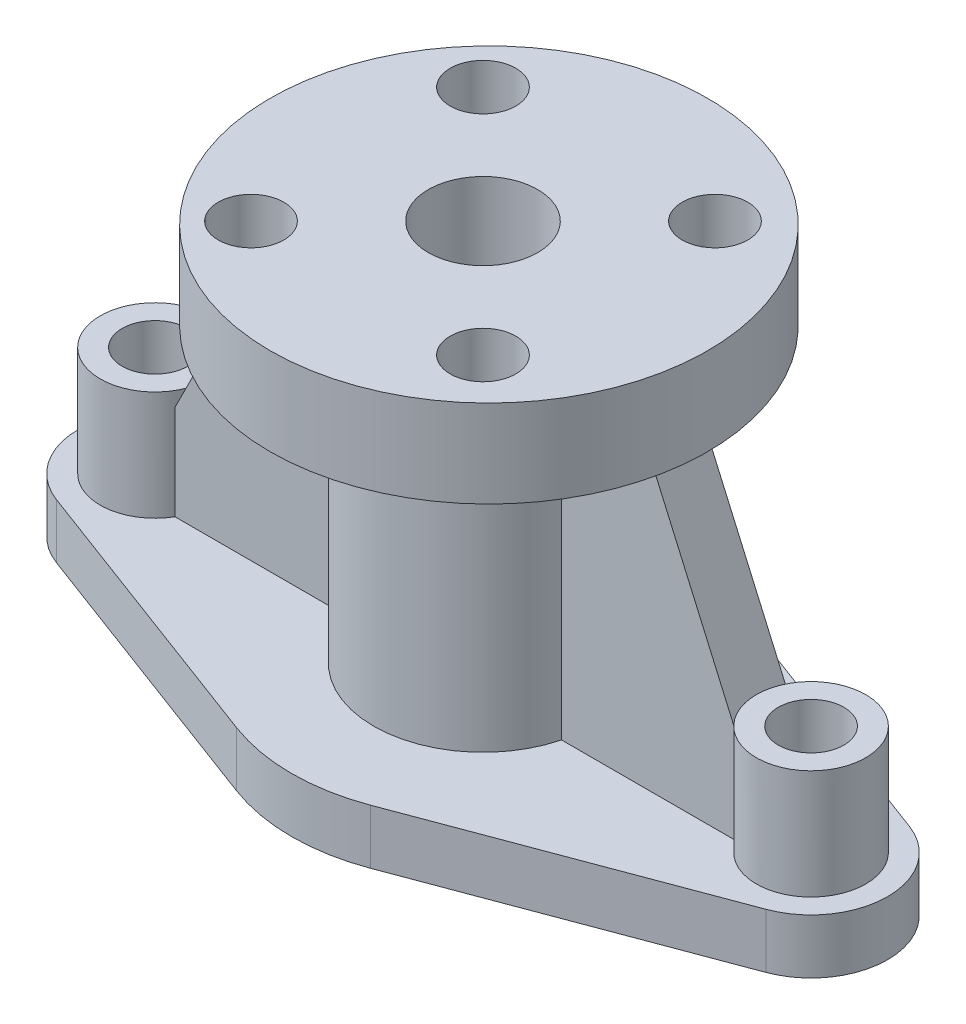
ISO-10303-21;
HEADER;
FILE_DESCRIPTION(('STEP AP214'),'2;1');
FILE_NAME('part.step','',(''),(''),'','','');
FILE_SCHEMA(('AUTOMOTIVE_DESIGN { 1 0 10303 214 1 1 1 1 }'));
ENDSEC;
DATA;
#1=APPLICATION_CONTEXT('core data for automotive mechanical design processes');
#2=APPLICATION_PROTOCOL_DEFINITION('international standard','automotive_design',2000,#1);
#3=PRODUCT_CONTEXT('',#1,'mechanical');
#4=PRODUCT('Part','Part','',(#3));
#5=PRODUCT_RELATED_PRODUCT_CATEGORY('part','',(#4));
#6=PRODUCT_DEFINITION_FORMATION('','',#4);
#7=PRODUCT_DEFINITION_CONTEXT('part definition',#1,'design');
#8=PRODUCT_DEFINITION('design','',#6,#7);
#9=PRODUCT_DEFINITION_SHAPE('','',#8);
#10=(LENGTH_UNIT() NAMED_UNIT(*) SI_UNIT(.MILLI.,.METRE.));
#11=(NAMED_UNIT(*) PLANE_ANGLE_UNIT() SI_UNIT($,.RADIAN.));
#12=(NAMED_UNIT(*) SI_UNIT($,.STERADIAN.) SOLID_ANGLE_UNIT());
#13=UNCERTAINTY_MEASURE_WITH_UNIT(LENGTH_MEASURE(1.E-05),#10,'distance_accuracy_value','');
#14=(GEOMETRIC_REPRESENTATION_CONTEXT(3) GLOBAL_UNCERTAINTY_ASSIGNED_CONTEXT((#13)) GLOBAL_UNIT_ASSIGNED_CONTEXT((#10,
#11,#12)) REPRESENTATION_CONTEXT('',''));
#15=CARTESIAN_POINT('',(0.,0.,0.));
#16=DIRECTION('',(0.,0.,1.));
#17=DIRECTION('',(1.,0.,0.));
#18=AXIS2_PLACEMENT_3D('',#15,#16,#17);
#19=CARTESIAN_POINT('',(0.,-0.002000000000002,0.));
#20=DIRECTION('',(0.,1.,0.));
#21=DIRECTION('',(0.,0.,1.));
#22=AXIS2_PLACEMENT_3D('',#19,#20,#21);
#23=CYLINDRICAL_SURFACE('',#22,20.);
#24=DIRECTION('',(0.,1.,0.));
#25=VECTOR('',#24,1.);
#26=CARTESIAN_POINT('',(19.3649167310371,-0.002000000000002,-5.));
#27=LINE('',#26,#25);
#28=CARTESIAN_POINT('',(19.3649167310371,10.,-5.));
#29=VERTEX_POINT('',#28);
#30=CARTESIAN_POINT('',(19.3649167310371,64.,-5.));
#31=VERTEX_POINT('',#30);
#32=EDGE_CURVE('E191',#29,#31,#27,.T.);
#33=ORIENTED_EDGE('',*,*,#32,.F.);
#34=CARTESIAN_POINT('',(0.,10.,0.));
#35=DIRECTION('',(0.,1.,0.));
#36=DIRECTION('',(0.,0.,1.));
#37=AXIS2_PLACEMENT_3D('',#34,#35,#36);
#38=CIRCLE('',#37,20.);
#39=CARTESIAN_POINT('',(-19.3649167310371,10.,-5.));
#40=VERTEX_POINT('',#39);
#41=EDGE_CURVE('E265',#29,#40,#38,.T.);
#42=ORIENTED_EDGE('',*,*,#41,.T.);
#43=DIRECTION('',(0.,1.,0.));
#44=VECTOR('',#43,1.);
#45=CARTESIAN_POINT('',(-19.3649167310371,-0.002000000000002,-5.));
#46=LINE('',#45,#44);
#47=CARTESIAN_POINT('',(-19.3649167310371,64.,-5.));
#48=VERTEX_POINT('',#47);
#49=EDGE_CURVE('E228',#48,#40,#46,.F.);
#50=ORIENTED_EDGE('',*,*,#49,.F.);
#51=CARTESIAN_POINT('',(0.,64.,0.));
#52=DIRECTION('',(0.,-1.,0.));
#53=DIRECTION('',(0.,0.,-1.));
#54=AXIS2_PLACEMENT_3D('',#51,#52,#53);
#55=CIRCLE('',#54,20.);
#56=EDGE_CURVE('E261',#48,#31,#55,.T.);
#57=ORIENTED_EDGE('',*,*,#56,.T.);
#58=EDGE_LOOP('',(#33,#42,#50,#57));
#59=FACE_BOUND('',#58,.T.);
#60=ADVANCED_FACE('F39',(#59),#23,.T.);
#61=CARTESIAN_POINT('',(-60.,10.,0.));
#62=DIRECTION('',(0.,-1.,0.));
#63=DIRECTION('',(0.,0.,-1.));
#64=AXIS2_PLACEMENT_3D('',#61,#62,#63);
#65=CYLINDRICAL_SURFACE('',#64,14.);
#66=DIRECTION('',(0.,-1.,0.));
#67=VECTOR('',#66,1.);
#68=CARTESIAN_POINT('',(-64.9,10.,13.1144957966366));
#69=LINE('',#68,#67);
#70=CARTESIAN_POINT('',(-64.9,10.,13.1144957966366));
#71=VERTEX_POINT('',#70);
#72=CARTESIAN_POINT('',(-64.9,0.,13.1144957966366));
#73=VERTEX_POINT('',#72);
#74=EDGE_CURVE('E11',#71,#73,#69,.T.);
#75=ORIENTED_EDGE('',*,*,#74,.F.);
#76=CARTESIAN_POINT('',(-60.,10.,0.));
#77=DIRECTION('',(0.,1.,0.));
#78=DIRECTION('',(0.,0.,1.));
#79=AXIS2_PLACEMENT_3D('',#76,#77,#78);
#80=CIRCLE('',#79,14.);
#81=CARTESIAN_POINT('',(-64.9,10.,-13.1144957966366));
#82=VERTEX_POINT('',#81);
#83=EDGE_CURVE('E288',#82,#71,#80,.T.);
#84=ORIENTED_EDGE('',*,*,#83,.F.);
#85=DIRECTION('',(0.,-1.,0.));
#86=VECTOR('',#85,1.);
#87=CARTESIAN_POINT('',(-64.9,10.,-13.1144957966366));
#88=LINE('',#87,#86);
#89=CARTESIAN_POINT('',(-64.9,0.,-13.1144957966366));
#90=VERTEX_POINT('',#89);
#91=EDGE_CURVE('E303',#82,#90,#88,.T.);
#92=ORIENTED_EDGE('',*,*,#91,.T.);
#93=CARTESIAN_POINT('',(-60.,0.,0.));
#94=DIRECTION('',(0.,1.,0.));
#95=DIRECTION('',(0.,0.,1.));
#96=AXIS2_PLACEMENT_3D('',#93,#94,#95);
#97=CIRCLE('',#96,14.);
#98=EDGE_CURVE('E280',#90,#73,#97,.T.);
#99=ORIENTED_EDGE('',*,*,#98,.T.);
#100=EDGE_LOOP('',(#75,#84,#92,#99));
#101=FACE_BOUND('',#100,.T.);
#102=ADVANCED_FACE('F41',(#101),#65,.T.);
#103=CARTESIAN_POINT('',(-64.9,10.,13.1144957966366));
#104=DIRECTION('',(0.35,0.,-0.93674969975976));
#105=DIRECTION('',(-0.93674969975976,0.,-0.35));
#106=AXIS2_PLACEMENT_3D('',#103,#104,#105);
#107=PLANE('',#106);
#108=DIRECTION('',(0.93674969975976,0.,0.35));
#109=VECTOR('',#108,1.);
#110=CARTESIAN_POINT('',(-64.9,0.,13.1144957966366));
#111=LINE('',#110,#109);
#112=CARTESIAN_POINT('',(-12.25,0.,32.7862394915916));
#113=VERTEX_POINT('',#112);
#114=EDGE_CURVE('E304',#73,#113,#111,.T.);
#115=ORIENTED_EDGE('',*,*,#114,.T.);
#116=DIRECTION('',(0.,-1.,0.));
#117=VECTOR('',#116,1.);
#118=CARTESIAN_POINT('',(-12.25,10.,32.7862394915916));
#119=LINE('',#118,#117);
#120=CARTESIAN_POINT('',(-12.25,10.,32.7862394915916));
#121=VERTEX_POINT('',#120);
#122=EDGE_CURVE('E48',#121,#113,#119,.T.);
#123=ORIENTED_EDGE('',*,*,#122,.F.);
#124=DIRECTION('',(0.93674969975976,0.,0.35));
#125=VECTOR('',#124,1.);
#126=CARTESIAN_POINT('',(-64.9,10.,13.1144957966366));
#127=LINE('',#126,#125);
#128=EDGE_CURVE('E286',#71,#121,#127,.T.);
#129=ORIENTED_EDGE('',*,*,#128,.F.);
#130=ORIENTED_EDGE('',*,*,#74,.T.);
#131=EDGE_LOOP('',(#115,#123,#129,#130));
#132=FACE_BOUND('',#131,.T.);
#133=ADVANCED_FACE('F362',(#132),#107,.F.);
#134=CARTESIAN_POINT('',(0.,10.,0.));
#135=DIRECTION('',(0.,-1.,0.));
#136=DIRECTION('',(0.,0.,-1.));
#137=AXIS2_PLACEMENT_3D('',#134,#135,#136);
#138=CYLINDRICAL_SURFACE('',#137,35.);
#139=CARTESIAN_POINT('',(0.,0.,0.));
#140=DIRECTION('',(0.,1.,0.));
#141=DIRECTION('',(0.,0.,1.));
#142=AXIS2_PLACEMENT_3D('',#139,#140,#141);
#143=CIRCLE('',#142,35.);
#144=CARTESIAN_POINT('',(12.25,0.,32.7862394915916));
#145=VERTEX_POINT('',#144);
#146=EDGE_CURVE('E310',#113,#145,#143,.T.);
#147=ORIENTED_EDGE('',*,*,#146,.T.);
#148=DIRECTION('',(0.,-1.,0.));
#149=VECTOR('',#148,1.);
#150=CARTESIAN_POINT('',(12.25,10.,32.7862394915916));
#151=LINE('',#150,#149);
#152=CARTESIAN_POINT('',(12.25,10.,32.7862394915916));
#153=VERTEX_POINT('',#152);
#154=EDGE_CURVE('E335',#153,#145,#151,.T.);
#155=ORIENTED_EDGE('',*,*,#154,.F.);
#156=CARTESIAN_POINT('',(0.,10.,0.));
#157=DIRECTION('',(0.,1.,0.));
#158=DIRECTION('',(0.,0.,1.));
#159=AXIS2_PLACEMENT_3D('',#156,#157,#158);
#160=CIRCLE('',#159,35.);
#161=EDGE_CURVE('E293',#121,#153,#160,.T.);
#162=ORIENTED_EDGE('',*,*,#161,.F.);
#163=ORIENTED_EDGE('',*,*,#122,.T.);
#164=EDGE_LOOP('',(#147,#155,#162,#163));
#165=FACE_BOUND('',#164,.T.);
#166=ADVANCED_FACE('F338',(#165),#138,.T.);
#167=CARTESIAN_POINT('',(64.9,10.,13.1144957966366));
#168=DIRECTION('',(-0.35,0.,-0.93674969975976));
#169=DIRECTION('',(-0.93674969975976,0.,0.35));
#170=AXIS2_PLACEMENT_3D('',#167,#168,#169);
#171=PLANE('',#170);
#172=DIRECTION('',(0.93674969975976,0.,-0.35));
#173=VECTOR('',#172,1.);
#174=CARTESIAN_POINT('',(64.9,0.,13.1144957966366));
#175=LINE('',#174,#173);
#176=CARTESIAN_POINT('',(64.9,0.,13.1144957966366));
#177=VERTEX_POINT('',#176);
#178=EDGE_CURVE('E307',#145,#177,#175,.T.);
#179=ORIENTED_EDGE('',*,*,#178,.T.);
#180=DIRECTION('',(0.,-1.,0.));
#181=VECTOR('',#180,1.);
#182=CARTESIAN_POINT('',(64.9,10.,13.1144957966366));
#183=LINE('',#182,#181);
#184=CARTESIAN_POINT('',(64.9,10.,13.1144957966366));
#185=VERTEX_POINT('',#184);
#186=EDGE_CURVE('E327',#185,#177,#183,.T.);
#187=ORIENTED_EDGE('',*,*,#186,.F.);
#188=DIRECTION('',(0.93674969975976,0.,-0.35));
#189=VECTOR('',#188,1.);
#190=CARTESIAN_POINT('',(64.9,10.,13.1144957966366));
#191=LINE('',#190,#189);
#192=EDGE_CURVE('E291',#153,#185,#191,.T.);
#193=ORIENTED_EDGE('',*,*,#192,.F.);
#194=ORIENTED_EDGE('',*,*,#154,.T.);
#195=EDGE_LOOP('',(#179,#187,#193,#194));
#196=FACE_BOUND('',#195,.T.);
#197=ADVANCED_FACE('F351',(#196),#171,.F.);
#198=CARTESIAN_POINT('',(60.,10.,0.));
#199=DIRECTION('',(0.,-1.,0.));
#200=DIRECTION('',(0.,0.,-1.));
#201=AXIS2_PLACEMENT_3D('',#198,#199,#200);
#202=CYLINDRICAL_SURFACE('',#201,14.);
#203=CARTESIAN_POINT('',(60.,0.,0.));
#204=DIRECTION('',(0.,1.,0.));
#205=DIRECTION('',(0.,0.,1.));
#206=AXIS2_PLACEMENT_3D('',#203,#204,#205);
#207=CIRCLE('',#206,14.);
#208=CARTESIAN_POINT('',(64.9,0.,-13.1144957966367));
#209=VERTEX_POINT('',#208);
#210=EDGE_CURVE('E311',#177,#209,#207,.T.);
#211=ORIENTED_EDGE('',*,*,#210,.T.);
#212=DIRECTION('',(0.,-1.,0.));
#213=VECTOR('',#212,1.);
#214=CARTESIAN_POINT('',(64.9,10.,-13.1144957966367));
#215=LINE('',#214,#213);
#216=CARTESIAN_POINT('',(64.9,10.,-13.1144957966367));
#217=VERTEX_POINT('',#216);
#218=EDGE_CURVE('E328',#217,#209,#215,.T.);
#219=ORIENTED_EDGE('',*,*,#218,.F.);
#220=CARTESIAN_POINT('',(60.,10.,0.));
#221=DIRECTION('',(0.,1.,0.));
#222=DIRECTION('',(0.,0.,1.));
#223=AXIS2_PLACEMENT_3D('',#220,#221,#222);
#224=CIRCLE('',#223,14.);
#225=EDGE_CURVE('E294',#185,#217,#224,.T.);
#226=ORIENTED_EDGE('',*,*,#225,.F.);
#227=ORIENTED_EDGE('',*,*,#186,.T.);
#228=EDGE_LOOP('',(#211,#219,#226,#227));
#229=FACE_BOUND('',#228,.T.);
#230=ADVANCED_FACE('F357',(#229),#202,.T.);
#231=CARTESIAN_POINT('',(64.9,10.,-13.1144957966367));
#232=DIRECTION('',(-0.35,0.,0.93674969975976));
#233=DIRECTION('',(0.93674969975976,0.,0.35));
#234=AXIS2_PLACEMENT_3D('',#231,#232,#233);
#235=PLANE('',#234);
#236=DIRECTION('',(-0.93674969975976,0.,-0.35));
#237=VECTOR('',#236,1.);
#238=CARTESIAN_POINT('',(64.9,0.,-13.1144957966367));
#239=LINE('',#238,#237);
#240=CARTESIAN_POINT('',(12.25,0.,-32.7862394915916));
#241=VERTEX_POINT('',#240);
#242=EDGE_CURVE('E312',#209,#241,#239,.T.);
#243=ORIENTED_EDGE('',*,*,#242,.T.);
#244=DIRECTION('',(0.,-1.,0.));
#245=VECTOR('',#244,1.);
#246=CARTESIAN_POINT('',(12.25,10.,-32.7862394915916));
#247=LINE('',#246,#245);
#248=CARTESIAN_POINT('',(12.25,10.,-32.7862394915916));
#249=VERTEX_POINT('',#248);
#250=EDGE_CURVE('E325',#249,#241,#247,.T.);
#251=ORIENTED_EDGE('',*,*,#250,.F.);
#252=DIRECTION('',(-0.93674969975976,0.,-0.35));
#253=VECTOR('',#252,1.);
#254=CARTESIAN_POINT('',(64.9,10.,-13.1144957966367));
#255=LINE('',#254,#253);
#256=EDGE_CURVE('E300',#217,#249,#255,.T.);
#257=ORIENTED_EDGE('',*,*,#256,.F.);
#258=ORIENTED_EDGE('',*,*,#218,.T.);
#259=EDGE_LOOP('',(#243,#251,#257,#258));
#260=FACE_BOUND('',#259,.T.);
#261=ADVANCED_FACE('F377',(#260),#235,.F.);
#262=CARTESIAN_POINT('',(0.,10.,0.));
#263=DIRECTION('',(0.,-1.,0.));
#264=DIRECTION('',(0.,0.,-1.));
#265=AXIS2_PLACEMENT_3D('',#262,#263,#264);
#266=CYLINDRICAL_SURFACE('',#265,35.);
#267=CARTESIAN_POINT('',(0.,0.,0.));
#268=DIRECTION('',(0.,1.,0.));
#269=DIRECTION('',(0.,0.,1.));
#270=AXIS2_PLACEMENT_3D('',#267,#268,#269);
#271=CIRCLE('',#270,35.);
#272=CARTESIAN_POINT('',(-12.25,0.,-32.7862394915916));
#273=VERTEX_POINT('',#272);
#274=EDGE_CURVE('E314',#241,#273,#271,.T.);
#275=ORIENTED_EDGE('',*,*,#274,.T.);
#276=DIRECTION('',(0.,-1.,0.));
#277=VECTOR('',#276,1.);
#278=CARTESIAN_POINT('',(-12.25,10.,-32.7862394915916));
#279=LINE('',#278,#277);
#280=CARTESIAN_POINT('',(-12.25,10.,-32.7862394915916));
#281=VERTEX_POINT('',#280);
#282=EDGE_CURVE('E318',#281,#273,#279,.T.);
#283=ORIENTED_EDGE('',*,*,#282,.F.);
#284=CARTESIAN_POINT('',(0.,10.,0.));
#285=DIRECTION('',(0.,1.,0.));
#286=DIRECTION('',(0.,0.,1.));
#287=AXIS2_PLACEMENT_3D('',#284,#285,#286);
#288=CIRCLE('',#287,35.);
#289=EDGE_CURVE('E299',#249,#281,#288,.T.);
#290=ORIENTED_EDGE('',*,*,#289,.F.);
#291=ORIENTED_EDGE('',*,*,#250,.T.);
#292=EDGE_LOOP('',(#275,#283,#290,#291));
#293=FACE_BOUND('',#292,.T.);
#294=ADVANCED_FACE('F376',(#293),#266,.T.);
#295=CARTESIAN_POINT('',(-64.9,10.,-13.1144957966366));
#296=DIRECTION('',(0.35,0.,0.93674969975976));
#297=DIRECTION('',(0.93674969975976,0.,-0.35));
#298=AXIS2_PLACEMENT_3D('',#295,#296,#297);
#299=PLANE('',#298);
#300=DIRECTION('',(-0.93674969975976,0.,0.35));
#301=VECTOR('',#300,1.);
#302=CARTESIAN_POINT('',(-64.9,0.,-13.1144957966366));
#303=LINE('',#302,#301);
#304=EDGE_CURVE('E289',#273,#90,#303,.T.);
#305=ORIENTED_EDGE('',*,*,#304,.T.);
#306=ORIENTED_EDGE('',*,*,#91,.F.);
#307=DIRECTION('',(-0.93674969975976,0.,0.35));
#308=VECTOR('',#307,1.);
#309=CARTESIAN_POINT('',(-64.9,10.,-13.1144957966366));
#310=LINE('',#309,#308);
#311=EDGE_CURVE('E301',#281,#82,#310,.T.);
#312=ORIENTED_EDGE('',*,*,#311,.F.);
#313=ORIENTED_EDGE('',*,*,#282,.T.);
#314=EDGE_LOOP('',(#305,#306,#312,#313));
#315=FACE_BOUND('',#314,.T.);
#316=ADVANCED_FACE('F371',(#315),#299,.F.);
#317=CARTESIAN_POINT('',(-60.,10.,0.));
#318=DIRECTION('',(0.,1.,0.));
#319=DIRECTION('',(0.,0.,1.));
#320=AXIS2_PLACEMENT_3D('',#317,#318,#319);
#321=PLANE('',#320);
#322=DIRECTION('',(1.,0.,0.));
#323=VECTOR('',#322,1.);
#324=CARTESIAN_POINT('',(-60.,10.,5.));
#325=LINE('',#324,#323);
#326=CARTESIAN_POINT('',(-51.3397459621556,10.,5.));
#327=VERTEX_POINT('',#326);
#328=CARTESIAN_POINT('',(-19.3649167310371,10.,5.));
#329=VERTEX_POINT('',#328);
#330=EDGE_CURVE('E237',#327,#329,#325,.T.);
#331=ORIENTED_EDGE('',*,*,#330,.F.);
#332=CARTESIAN_POINT('',(-60.,10.,0.));
#333=DIRECTION('',(0.,1.,0.));
#334=DIRECTION('',(0.,0.,1.));
#335=AXIS2_PLACEMENT_3D('',#332,#333,#334);
#336=CIRCLE('',#335,10.);
#337=CARTESIAN_POINT('',(-51.3397459621556,10.,-5.));
#338=VERTEX_POINT('',#337);
#339=EDGE_CURVE('E274',#338,#327,#336,.T.);
#340=ORIENTED_EDGE('',*,*,#339,.F.);
#341=DIRECTION('',(1.,0.,0.));
#342=VECTOR('',#341,1.);
#343=CARTESIAN_POINT('',(-60.,10.,-5.));
#344=LINE('',#343,#342);
#345=EDGE_CURVE('E227',#338,#40,#344,.T.);
#346=ORIENTED_EDGE('',*,*,#345,.T.);
#347=ORIENTED_EDGE('',*,*,#41,.F.);
#348=DIRECTION('',(1.,0.,0.));
#349=VECTOR('',#348,1.);
#350=CARTESIAN_POINT('',(-60.,10.,-5.));
#351=LINE('',#350,#349);
#352=CARTESIAN_POINT('',(51.3397459621556,10.,-5.));
#353=VERTEX_POINT('',#352);
#354=EDGE_CURVE('E207',#29,#353,#351,.T.);
#355=ORIENTED_EDGE('',*,*,#354,.T.);
#356=CARTESIAN_POINT('',(60.,10.,0.));
#357=DIRECTION('',(0.,1.,0.));
#358=DIRECTION('',(0.,0.,1.));
#359=AXIS2_PLACEMENT_3D('',#356,#357,#358);
#360=CIRCLE('',#359,9.99999999999999);
#361=CARTESIAN_POINT('',(51.3397459621556,10.,5.));
#362=VERTEX_POINT('',#361);
#363=EDGE_CURVE('E277',#362,#353,#360,.T.);
#364=ORIENTED_EDGE('',*,*,#363,.F.);
#365=DIRECTION('',(1.,0.,0.));
#366=VECTOR('',#365,1.);
#367=CARTESIAN_POINT('',(-60.,10.,5.));
#368=LINE('',#367,#366);
#369=CARTESIAN_POINT('',(19.3649167310371,10.,5.));
#370=VERTEX_POINT('',#369);
#371=EDGE_CURVE('E211',#370,#362,#368,.T.);
#372=ORIENTED_EDGE('',*,*,#371,.F.);
#373=EDGE_CURVE('E260',#329,#370,#38,.T.);
#374=ORIENTED_EDGE('',*,*,#373,.F.);
#375=EDGE_LOOP('',(#331,#340,#346,#347,#355,#364,#372,#374));
#376=FACE_BOUND('',#375,.T.);
#377=ORIENTED_EDGE('',*,*,#83,.T.);
#378=ORIENTED_EDGE('',*,*,#128,.T.);
#379=ORIENTED_EDGE('',*,*,#161,.T.);
#380=ORIENTED_EDGE('',*,*,#192,.T.);
#381=ORIENTED_EDGE('',*,*,#225,.T.);
#382=ORIENTED_EDGE('',*,*,#256,.T.);
#383=ORIENTED_EDGE('',*,*,#289,.T.);
#384=ORIENTED_EDGE('',*,*,#311,.T.);
#385=EDGE_LOOP('',(#377,#378,#379,#380,#381,#382,#383,#384));
#386=FACE_BOUND('',#385,.T.);
#387=ADVANCED_FACE('F363',(#376,#386),#321,.T.);
#388=CARTESIAN_POINT('',(-60.,0.,0.));
#389=DIRECTION('',(0.,1.,0.));
#390=DIRECTION('',(0.,0.,1.));
#391=AXIS2_PLACEMENT_3D('',#388,#389,#390);
#392=PLANE('',#391);
#393=CARTESIAN_POINT('',(0.,0.,0.));
#394=DIRECTION('',(0.,1.,0.));
#395=DIRECTION('',(0.,0.,1.));
#396=AXIS2_PLACEMENT_3D('',#393,#394,#395);
#397=CIRCLE('',#396,5.);
#398=CARTESIAN_POINT('',(0.,0.,5.));
#399=VERTEX_POINT('',#398);
#400=EDGE_CURVE('E635',#399,#399,#397,.T.);
#401=ORIENTED_EDGE('',*,*,#400,.T.);
#402=EDGE_LOOP('',(#401));
#403=FACE_BOUND('',#402,.T.);
#404=CARTESIAN_POINT('',(-60.,0.,0.));
#405=DIRECTION('',(0.,1.,0.));
#406=DIRECTION('',(0.,0.,1.));
#407=AXIS2_PLACEMENT_3D('',#404,#405,#406);
#408=CIRCLE('',#407,6.);
#409=CARTESIAN_POINT('',(-60.,0.,6.));
#410=VERTEX_POINT('',#409);
#411=EDGE_CURVE('E263',#410,#410,#408,.T.);
#412=ORIENTED_EDGE('',*,*,#411,.T.);
#413=EDGE_LOOP('',(#412));
#414=FACE_BOUND('',#413,.T.);
#415=CARTESIAN_POINT('',(60.,0.,0.));
#416=DIRECTION('',(0.,1.,0.));
#417=DIRECTION('',(0.,0.,1.));
#418=AXIS2_PLACEMENT_3D('',#415,#416,#417);
#419=CIRCLE('',#418,6.);
#420=CARTESIAN_POINT('',(60.,0.,5.99999999999998));
#421=VERTEX_POINT('',#420);
#422=EDGE_CURVE('E264',#421,#421,#419,.T.);
#423=ORIENTED_EDGE('',*,*,#422,.T.);
#424=EDGE_LOOP('',(#423));
#425=FACE_BOUND('',#424,.T.);
#426=ORIENTED_EDGE('',*,*,#114,.F.);
#427=ORIENTED_EDGE('',*,*,#98,.F.);
#428=ORIENTED_EDGE('',*,*,#304,.F.);
#429=ORIENTED_EDGE('',*,*,#274,.F.);
#430=ORIENTED_EDGE('',*,*,#242,.F.);
#431=ORIENTED_EDGE('',*,*,#210,.F.);
#432=ORIENTED_EDGE('',*,*,#178,.F.);
#433=ORIENTED_EDGE('',*,*,#146,.F.);
#434=EDGE_LOOP('',(#426,#427,#428,#429,#430,#431,#432,#433));
#435=FACE_BOUND('',#434,.T.);
#436=ADVANCED_FACE('F350',(#403,#414,#425,#435),#392,.F.);
#437=CARTESIAN_POINT('',(60.,30.,0.));
#438=DIRECTION('',(0.,1.,0.));
#439=DIRECTION('',(0.,0.,1.));
#440=AXIS2_PLACEMENT_3D('',#437,#438,#439);
#441=PLANE('',#440);
#442=CARTESIAN_POINT('',(60.,30.,0.));
#443=DIRECTION('',(0.,1.,0.));
#444=DIRECTION('',(0.,0.,1.));
#445=AXIS2_PLACEMENT_3D('',#442,#443,#444);
#446=CIRCLE('',#445,6.);
#447=CARTESIAN_POINT('',(60.,30.,5.99999999999998));
#448=VERTEX_POINT('',#447);
#449=EDGE_CURVE('E273',#448,#448,#446,.T.);
#450=ORIENTED_EDGE('',*,*,#449,.F.);
#451=EDGE_LOOP('',(#450));
#452=FACE_BOUND('',#451,.T.);
#453=CARTESIAN_POINT('',(60.,30.,0.));
#454=DIRECTION('',(0.,1.,0.));
#455=DIRECTION('',(0.,0.,1.));
#456=AXIS2_PLACEMENT_3D('',#453,#454,#455);
#457=CIRCLE('',#456,9.99999999999999);
#458=CARTESIAN_POINT('',(50.,30.,0.));
#459=VERTEX_POINT('',#458);
#460=EDGE_CURVE('E266',#459,#459,#457,.T.);
#461=ORIENTED_EDGE('',*,*,#460,.T.);
#462=EDGE_LOOP('',(#461));
#463=FACE_BOUND('',#462,.T.);
#464=ADVANCED_FACE('F453',(#452,#463),#441,.T.);
#465=CARTESIAN_POINT('',(60.,30.,0.));
#466=DIRECTION('',(0.,-1.,0.));
#467=DIRECTION('',(0.,0.,-1.));
#468=AXIS2_PLACEMENT_3D('',#465,#466,#467);
#469=CYLINDRICAL_SURFACE('',#468,9.99999999999999);
#470=CARTESIAN_POINT('',(60.,7.21626759204642,0.));
#471=DIRECTION('',(-0.915682698749412,-0.401901972141209,0.));
#472=DIRECTION('',(0.401901972141209,-0.915682698749412,0.));
#473=AXIS2_PLACEMENT_3D('',#470,#471,#472);
#474=ELLIPSE('',#473,24.8816893003115,9.99999999999999);
#475=CARTESIAN_POINT('',(51.3397459621556,26.947558650361,5.));
#476=VERTEX_POINT('',#475);
#477=EDGE_CURVE('E54',#459,#476,#474,.F.);
#478=ORIENTED_EDGE('',*,*,#477,.T.);
#479=DIRECTION('',(0.,-1.,0.));
#480=VECTOR('',#479,1.);
#481=CARTESIAN_POINT('',(51.3397459621556,30.,5.));
#482=LINE('',#481,#480);
#483=EDGE_CURVE('E183',#476,#362,#482,.T.);
#484=ORIENTED_EDGE('',*,*,#483,.T.);
#485=ORIENTED_EDGE('',*,*,#363,.T.);
#486=DIRECTION('',(0.,-1.,0.));
#487=VECTOR('',#486,1.);
#488=CARTESIAN_POINT('',(51.3397459621556,30.,-5.));
#489=LINE('',#488,#487);
#490=CARTESIAN_POINT('',(51.3397459621556,26.947558650361,-5.));
#491=VERTEX_POINT('',#490);
#492=EDGE_CURVE('E61',#491,#353,#489,.T.);
#493=ORIENTED_EDGE('',*,*,#492,.F.);
#494=EDGE_CURVE('E198',#491,#459,#474,.F.);
#495=ORIENTED_EDGE('',*,*,#494,.T.);
#496=ORIENTED_EDGE('',*,*,#460,.F.);
#497=EDGE_LOOP('',(#478,#484,#485,#493,#495,#496));
#498=FACE_BOUND('',#497,.T.);
#499=ADVANCED_FACE('F418',(#498),#469,.T.);
#500=CARTESIAN_POINT('',(60.,30.,0.));
#501=DIRECTION('',(0.,-1.,0.));
#502=DIRECTION('',(0.,0.,-1.));
#503=AXIS2_PLACEMENT_3D('',#500,#501,#502);
#504=CYLINDRICAL_SURFACE('',#503,6.);
#505=ORIENTED_EDGE('',*,*,#422,.F.);
#506=EDGE_LOOP('',(#505));
#507=FACE_BOUND('',#506,.T.);
#508=ORIENTED_EDGE('',*,*,#449,.T.);
#509=EDGE_LOOP('',(#508));
#510=FACE_BOUND('',#509,.T.);
#511=ADVANCED_FACE('F439',(#507,#510),#504,.F.);
#512=CARTESIAN_POINT('',(-60.,30.,0.));
#513=DIRECTION('',(0.,1.,0.));
#514=DIRECTION('',(0.,0.,1.));
#515=AXIS2_PLACEMENT_3D('',#512,#513,#514);
#516=PLANE('',#515);
#517=CARTESIAN_POINT('',(-60.,30.,0.));
#518=DIRECTION('',(0.,1.,0.));
#519=DIRECTION('',(0.,0.,1.));
#520=AXIS2_PLACEMENT_3D('',#517,#518,#519);
#521=CIRCLE('',#520,6.);
#522=CARTESIAN_POINT('',(-60.,30.,6.));
#523=VERTEX_POINT('',#522);
#524=EDGE_CURVE('E272',#523,#523,#521,.T.);
#525=ORIENTED_EDGE('',*,*,#524,.F.);
#526=EDGE_LOOP('',(#525));
#527=FACE_BOUND('',#526,.T.);
#528=CARTESIAN_POINT('',(-60.,30.,0.));
#529=DIRECTION('',(0.,1.,0.));
#530=DIRECTION('',(0.,0.,1.));
#531=AXIS2_PLACEMENT_3D('',#528,#529,#530);
#532=CIRCLE('',#531,10.);
#533=CARTESIAN_POINT('',(-50.,30.,0.));
#534=VERTEX_POINT('',#533);
#535=EDGE_CURVE('E279',#534,#534,#532,.T.);
#536=ORIENTED_EDGE('',*,*,#535,.T.);
#537=EDGE_LOOP('',(#536));
#538=FACE_BOUND('',#537,.T.);
#539=ADVANCED_FACE('F438',(#527,#538),#516,.T.);
#540=CARTESIAN_POINT('',(-60.,30.,0.));
#541=DIRECTION('',(0.,-1.,0.));
#542=DIRECTION('',(0.,0.,-1.));
#543=AXIS2_PLACEMENT_3D('',#540,#541,#542);
#544=CYLINDRICAL_SURFACE('',#543,10.);
#545=CARTESIAN_POINT('',(-60.,10.0902636301007,0.));
#546=DIRECTION('',(-0.893615456318118,0.448833394735019,0.));
#547=DIRECTION('',(-0.448833394735019,-0.893615456318118,0.));
#548=AXIS2_PLACEMENT_3D('',#545,#546,#547);
#549=ELLIPSE('',#548,22.2799820987112,10.);
#550=CARTESIAN_POINT('',(-51.3397459621556,27.3326011090845,-5.));
#551=VERTEX_POINT('',#550);
#552=EDGE_CURVE('E247',#534,#551,#549,.T.);
#553=ORIENTED_EDGE('',*,*,#552,.T.);
#554=DIRECTION('',(0.,-1.,0.));
#555=VECTOR('',#554,1.);
#556=CARTESIAN_POINT('',(-51.3397459621556,30.,-5.));
#557=LINE('',#556,#555);
#558=EDGE_CURVE('E229',#338,#551,#557,.F.);
#559=ORIENTED_EDGE('',*,*,#558,.F.);
#560=ORIENTED_EDGE('',*,*,#339,.T.);
#561=DIRECTION('',(0.,-1.,0.));
#562=VECTOR('',#561,1.);
#563=CARTESIAN_POINT('',(-51.3397459621556,30.,5.));
#564=LINE('',#563,#562);
#565=CARTESIAN_POINT('',(-51.3397459621556,27.3326011090845,5.));
#566=VERTEX_POINT('',#565);
#567=EDGE_CURVE('E245',#327,#566,#564,.F.);
#568=ORIENTED_EDGE('',*,*,#567,.T.);
#569=EDGE_CURVE('E249',#566,#534,#549,.T.);
#570=ORIENTED_EDGE('',*,*,#569,.T.);
#571=ORIENTED_EDGE('',*,*,#535,.F.);
#572=EDGE_LOOP('',(#553,#559,#560,#568,#570,#571));
#573=FACE_BOUND('',#572,.T.);
#574=ADVANCED_FACE('F406',(#573),#544,.T.);
#575=CARTESIAN_POINT('',(-60.,30.,0.));
#576=DIRECTION('',(0.,-1.,0.));
#577=DIRECTION('',(0.,0.,-1.));
#578=AXIS2_PLACEMENT_3D('',#575,#576,#577);
#579=CYLINDRICAL_SURFACE('',#578,6.);
#580=ORIENTED_EDGE('',*,*,#411,.F.);
#581=EDGE_LOOP('',(#580));
#582=FACE_BOUND('',#581,.T.);
#583=ORIENTED_EDGE('',*,*,#524,.T.);
#584=EDGE_LOOP('',(#583));
#585=FACE_BOUND('',#584,.T.);
#586=ADVANCED_FACE('F397',(#582,#585),#579,.F.);
#587=ORIENTED_EDGE('',*,*,#373,.T.);
#588=DIRECTION('',(0.,1.,0.));
#589=VECTOR('',#588,1.);
#590=CARTESIAN_POINT('',(19.3649167310371,-0.002000000000002,5.));
#591=LINE('',#590,#589);
#592=CARTESIAN_POINT('',(19.3649167310371,64.,5.));
#593=VERTEX_POINT('',#592);
#594=EDGE_CURVE('E208',#370,#593,#591,.T.);
#595=ORIENTED_EDGE('',*,*,#594,.T.);
#596=CARTESIAN_POINT('',(-19.3649167310371,64.,5.));
#597=VERTEX_POINT('',#596);
#598=EDGE_CURVE('E251',#593,#597,#55,.T.);
#599=ORIENTED_EDGE('',*,*,#598,.T.);
#600=DIRECTION('',(0.,1.,0.));
#601=VECTOR('',#600,1.);
#602=CARTESIAN_POINT('',(-19.3649167310371,-0.002000000000002,5.));
#603=LINE('',#602,#601);
#604=EDGE_CURVE('E238',#597,#329,#603,.F.);
#605=ORIENTED_EDGE('',*,*,#604,.T.);
#606=EDGE_LOOP('',(#587,#595,#599,#605));
#607=FACE_BOUND('',#606,.T.);
#608=ADVANCED_FACE('F393',(#607),#23,.T.);
#609=CARTESIAN_POINT('',(1.07707192517284,64.,0.));
#610=DIRECTION('',(0.,1.,0.));
#611=DIRECTION('',(0.,0.,1.));
#612=AXIS2_PLACEMENT_3D('',#609,#610,#611);
#613=CYLINDRICAL_SURFACE('',#612,40.);
#614=CARTESIAN_POINT('',(1.07707192517284,80.,0.));
#615=DIRECTION('',(0.,1.,0.));
#616=DIRECTION('',(0.,0.,1.));
#617=AXIS2_PLACEMENT_3D('',#614,#615,#616);
#618=CIRCLE('',#617,40.);
#619=CARTESIAN_POINT('',(1.07707192517284,80.,40.));
#620=VERTEX_POINT('',#619);
#621=EDGE_CURVE('E253',#620,#620,#618,.T.);
#622=ORIENTED_EDGE('',*,*,#621,.F.);
#623=EDGE_LOOP('',(#622));
#624=FACE_BOUND('',#623,.T.);
#625=CARTESIAN_POINT('',(1.07707192517284,64.,0.));
#626=DIRECTION('',(0.,1.,0.));
#627=DIRECTION('',(0.,0.,1.));
#628=AXIS2_PLACEMENT_3D('',#625,#626,#627);
#629=CIRCLE('',#628,40.);
#630=CARTESIAN_POINT('',(1.07707192517284,64.,40.));
#631=VERTEX_POINT('',#630);
#632=EDGE_CURVE('E252',#631,#631,#629,.T.);
#633=ORIENTED_EDGE('',*,*,#632,.T.);
#634=EDGE_LOOP('',(#633));
#635=FACE_BOUND('',#634,.T.);
#636=ADVANCED_FACE('F399',(#624,#635),#613,.T.);
#637=CARTESIAN_POINT('',(1.07707192517284,64.,0.));
#638=DIRECTION('',(0.,1.,0.));
#639=DIRECTION('',(0.,0.,1.));
#640=AXIS2_PLACEMENT_3D('',#637,#638,#639);
#641=PLANE('',#640);
#642=CARTESIAN_POINT('',(-21.2132034355967,64.,21.2132034355962));
#643=DIRECTION('',(0.,1.,0.));
#644=DIRECTION('',(0.,0.,1.));
#645=AXIS2_PLACEMENT_3D('',#642,#643,#644);
#646=CIRCLE('',#645,6.);
#647=CARTESIAN_POINT('',(-21.2132034355967,64.,27.2132034355962));
#648=VERTEX_POINT('',#647);
#649=EDGE_CURVE('E639',#648,#648,#646,.T.);
#650=ORIENTED_EDGE('',*,*,#649,.T.);
#651=EDGE_LOOP('',(#650));
#652=FACE_BOUND('',#651,.T.);
#653=CARTESIAN_POINT('',(21.2132034355962,64.,21.2132034355966));
#654=DIRECTION('',(0.,1.,0.));
#655=DIRECTION('',(0.,0.,1.));
#656=AXIS2_PLACEMENT_3D('',#653,#654,#655);
#657=CIRCLE('',#656,6.);
#658=CARTESIAN_POINT('',(21.2132034355962,64.,27.2132034355966));
#659=VERTEX_POINT('',#658);
#660=EDGE_CURVE('E641',#659,#659,#657,.T.);
#661=ORIENTED_EDGE('',*,*,#660,.T.);
#662=EDGE_LOOP('',(#661));
#663=FACE_BOUND('',#662,.T.);
#664=CARTESIAN_POINT('',(21.2132034355965,64.,-21.2132034355963));
#665=DIRECTION('',(0.,1.,0.));
#666=DIRECTION('',(0.,0.,1.));
#667=AXIS2_PLACEMENT_3D('',#664,#665,#666);
#668=CIRCLE('',#667,6.);
#669=CARTESIAN_POINT('',(21.2132034355965,64.,-15.2132034355963));
#670=VERTEX_POINT('',#669);
#671=EDGE_CURVE('E650',#670,#670,#668,.T.);
#672=ORIENTED_EDGE('',*,*,#671,.T.);
#673=EDGE_LOOP('',(#672));
#674=FACE_BOUND('',#673,.T.);
#675=CARTESIAN_POINT('',(-21.2132034355964,64.,-21.2132034355965));
#676=DIRECTION('',(0.,1.,0.));
#677=DIRECTION('',(0.,0.,1.));
#678=AXIS2_PLACEMENT_3D('',#675,#676,#677);
#679=CIRCLE('',#678,6.);
#680=CARTESIAN_POINT('',(-21.2132034355964,64.,-15.2132034355965));
#681=VERTEX_POINT('',#680);
#682=EDGE_CURVE('E636',#681,#681,#679,.T.);
#683=ORIENTED_EDGE('',*,*,#682,.T.);
#684=EDGE_LOOP('',(#683));
#685=FACE_BOUND('',#684,.T.);
#686=DIRECTION('',(0.,0.,1.));
#687=VECTOR('',#686,1.);
#688=CARTESIAN_POINT('',(-32.9229280748272,64.,0.));
#689=LINE('',#688,#687);
#690=CARTESIAN_POINT('',(-32.9229280748272,64.,-5.));
#691=VERTEX_POINT('',#690);
#692=CARTESIAN_POINT('',(-32.9229280748272,64.,5.));
#693=VERTEX_POINT('',#692);
#694=EDGE_CURVE('E246',#691,#693,#689,.T.);
#695=ORIENTED_EDGE('',*,*,#694,.T.);
#696=DIRECTION('',(1.,0.,0.));
#697=VECTOR('',#696,1.);
#698=CARTESIAN_POINT('',(1.07707192517284,64.,5.));
#699=LINE('',#698,#697);
#700=EDGE_CURVE('E232',#693,#597,#699,.T.);
#701=ORIENTED_EDGE('',*,*,#700,.T.);
#702=ORIENTED_EDGE('',*,*,#598,.F.);
#703=DIRECTION('',(1.,0.,0.));
#704=VECTOR('',#703,1.);
#705=CARTESIAN_POINT('',(1.07707192517284,64.,5.));
#706=LINE('',#705,#704);
#707=CARTESIAN_POINT('',(35.0770719251728,64.,5.));
#708=VERTEX_POINT('',#707);
#709=EDGE_CURVE('E177',#593,#708,#706,.T.);
#710=ORIENTED_EDGE('',*,*,#709,.T.);
#711=DIRECTION('',(0.,0.,1.));
#712=VECTOR('',#711,1.);
#713=CARTESIAN_POINT('',(35.0770719251728,64.,0.));
#714=LINE('',#713,#712);
#715=CARTESIAN_POINT('',(35.0770719251728,64.,-5.));
#716=VERTEX_POINT('',#715);
#717=EDGE_CURVE('E171',#708,#716,#714,.F.);
#718=ORIENTED_EDGE('',*,*,#717,.T.);
#719=DIRECTION('',(1.,0.,0.));
#720=VECTOR('',#719,1.);
#721=CARTESIAN_POINT('',(1.07707192517284,64.,-5.));
#722=LINE('',#721,#720);
#723=EDGE_CURVE('E174',#31,#716,#722,.T.);
#724=ORIENTED_EDGE('',*,*,#723,.F.);
#725=ORIENTED_EDGE('',*,*,#56,.F.);
#726=DIRECTION('',(1.,0.,0.));
#727=VECTOR('',#726,1.);
#728=CARTESIAN_POINT('',(1.07707192517284,64.,-5.));
#729=LINE('',#728,#727);
#730=EDGE_CURVE('E219',#691,#48,#729,.T.);
#731=ORIENTED_EDGE('',*,*,#730,.F.);
#732=EDGE_LOOP('',(#695,#701,#702,#710,#718,#724,#725,#731));
#733=FACE_BOUND('',#732,.T.);
#734=ORIENTED_EDGE('',*,*,#632,.F.);
#735=EDGE_LOOP('',(#734));
#736=FACE_BOUND('',#735,.T.);
#737=ADVANCED_FACE('F173',(#652,#663,#674,#685,#733,#736),#641,.F.);
#738=CARTESIAN_POINT('',(1.07707192517284,80.,0.));
#739=DIRECTION('',(0.,1.,0.));
#740=DIRECTION('',(0.,0.,1.));
#741=AXIS2_PLACEMENT_3D('',#738,#739,#740);
#742=PLANE('',#741);
#743=CARTESIAN_POINT('',(-21.2132034355967,80.,21.2132034355962));
#744=DIRECTION('',(0.,1.,0.));
#745=DIRECTION('',(0.,0.,1.));
#746=AXIS2_PLACEMENT_3D('',#743,#744,#745);
#747=CIRCLE('',#746,6.);
#748=CARTESIAN_POINT('',(-21.2132034355967,80.,27.2132034355962));
#749=VERTEX_POINT('',#748);
#750=EDGE_CURVE('E613',#749,#749,#747,.T.);
#751=ORIENTED_EDGE('',*,*,#750,.F.);
#752=EDGE_LOOP('',(#751));
#753=FACE_BOUND('',#752,.T.);
#754=CARTESIAN_POINT('',(21.2132034355962,80.,21.2132034355966));
#755=DIRECTION('',(0.,1.,0.));
#756=DIRECTION('',(0.,0.,1.));
#757=AXIS2_PLACEMENT_3D('',#754,#755,#756);
#758=CIRCLE('',#757,6.);
#759=CARTESIAN_POINT('',(21.2132034355962,80.,27.2132034355966));
#760=VERTEX_POINT('',#759);
#761=EDGE_CURVE('E612',#760,#760,#758,.T.);
#762=ORIENTED_EDGE('',*,*,#761,.F.);
#763=EDGE_LOOP('',(#762));
#764=FACE_BOUND('',#763,.T.);
#765=CARTESIAN_POINT('',(21.2132034355965,80.,-21.2132034355963));
#766=DIRECTION('',(0.,1.,0.));
#767=DIRECTION('',(0.,0.,1.));
#768=AXIS2_PLACEMENT_3D('',#765,#766,#767);
#769=CIRCLE('',#768,6.);
#770=CARTESIAN_POINT('',(21.2132034355965,80.,-15.2132034355963));
#771=VERTEX_POINT('',#770);
#772=EDGE_CURVE('E620',#771,#771,#769,.T.);
#773=ORIENTED_EDGE('',*,*,#772,.F.);
#774=EDGE_LOOP('',(#773));
#775=FACE_BOUND('',#774,.T.);
#776=CARTESIAN_POINT('',(-21.2132034355964,80.,-21.2132034355965));
#777=DIRECTION('',(0.,1.,0.));
#778=DIRECTION('',(0.,0.,1.));
#779=AXIS2_PLACEMENT_3D('',#776,#777,#778);
#780=CIRCLE('',#779,6.);
#781=CARTESIAN_POINT('',(-21.2132034355964,80.,-15.2132034355965));
#782=VERTEX_POINT('',#781);
#783=EDGE_CURVE('E621',#782,#782,#780,.T.);
#784=ORIENTED_EDGE('',*,*,#783,.F.);
#785=EDGE_LOOP('',(#784));
#786=FACE_BOUND('',#785,.T.);
#787=CARTESIAN_POINT('',(0.,80.,0.));
#788=DIRECTION('',(0.,1.,0.));
#789=DIRECTION('',(0.,0.,1.));
#790=AXIS2_PLACEMENT_3D('',#787,#788,#789);
#791=CIRCLE('',#790,10.);
#792=CARTESIAN_POINT('',(0.,80.,10.));
#793=VERTEX_POINT('',#792);
#794=EDGE_CURVE('E203',#793,#793,#791,.T.);
#795=ORIENTED_EDGE('',*,*,#794,.F.);
#796=EDGE_LOOP('',(#795));
#797=FACE_BOUND('',#796,.T.);
#798=ORIENTED_EDGE('',*,*,#621,.T.);
#799=EDGE_LOOP('',(#798));
#800=FACE_BOUND('',#799,.T.);
#801=ADVANCED_FACE('F485',(#753,#764,#775,#786,#797,#800),#742,.T.);
#802=CARTESIAN_POINT('',(-32.9229280748272,64.,0.));
#803=DIRECTION('',(-0.893615456318118,0.448833394735019,0.));
#804=DIRECTION('',(-0.448833394735019,-0.893615456318118,0.));
#805=AXIS2_PLACEMENT_3D('',#802,#803,#804);
#806=PLANE('',#805);
#807=ORIENTED_EDGE('',*,*,#569,.F.);
#808=DIRECTION('',(-0.448833394735019,-0.893615456318118,0.));
#809=VECTOR('',#808,1.);
#810=CARTESIAN_POINT('',(-32.9229280748272,64.,5.));
#811=LINE('',#810,#809);
#812=EDGE_CURVE('E220',#693,#566,#811,.T.);
#813=ORIENTED_EDGE('',*,*,#812,.F.);
#814=ORIENTED_EDGE('',*,*,#694,.F.);
#815=DIRECTION('',(-0.448833394735019,-0.893615456318118,0.));
#816=VECTOR('',#815,1.);
#817=CARTESIAN_POINT('',(-32.9229280748272,64.,-5.));
#818=LINE('',#817,#816);
#819=EDGE_CURVE('E223',#691,#551,#818,.T.);
#820=ORIENTED_EDGE('',*,*,#819,.T.);
#821=ORIENTED_EDGE('',*,*,#552,.F.);
#822=EDGE_LOOP('',(#807,#813,#814,#820,#821));
#823=FACE_BOUND('',#822,.T.);
#824=ADVANCED_FACE('F426',(#823),#806,.T.);
#825=CARTESIAN_POINT('',(0.,40.,5.));
#826=DIRECTION('',(0.,0.,1.));
#827=DIRECTION('',(1.,0.,0.));
#828=AXIS2_PLACEMENT_3D('',#825,#826,#827);
#829=PLANE('',#828);
#830=ORIENTED_EDGE('',*,*,#567,.F.);
#831=ORIENTED_EDGE('',*,*,#330,.T.);
#832=ORIENTED_EDGE('',*,*,#604,.F.);
#833=ORIENTED_EDGE('',*,*,#700,.F.);
#834=ORIENTED_EDGE('',*,*,#812,.T.);
#835=EDGE_LOOP('',(#830,#831,#832,#833,#834));
#836=FACE_BOUND('',#835,.T.);
#837=ADVANCED_FACE('F434',(#836),#829,.T.);
#838=CARTESIAN_POINT('',(0.,40.,-5.));
#839=DIRECTION('',(0.,0.,1.));
#840=DIRECTION('',(1.,0.,0.));
#841=AXIS2_PLACEMENT_3D('',#838,#839,#840);
#842=PLANE('',#841);
#843=ORIENTED_EDGE('',*,*,#345,.F.);
#844=ORIENTED_EDGE('',*,*,#558,.T.);
#845=ORIENTED_EDGE('',*,*,#819,.F.);
#846=ORIENTED_EDGE('',*,*,#730,.T.);
#847=ORIENTED_EDGE('',*,*,#49,.T.);
#848=EDGE_LOOP('',(#843,#844,#845,#846,#847));
#849=FACE_BOUND('',#848,.T.);
#850=ADVANCED_FACE('F427',(#849),#842,.F.);
#851=CARTESIAN_POINT('',(35.0770719251728,64.,0.));
#852=DIRECTION('',(-0.915682698749412,-0.401901972141209,0.));
#853=DIRECTION('',(0.401901972141209,-0.915682698749412,0.));
#854=AXIS2_PLACEMENT_3D('',#851,#852,#853);
#855=PLANE('',#854);
#856=ORIENTED_EDGE('',*,*,#494,.F.);
#857=DIRECTION('',(0.401901972141209,-0.915682698749412,0.));
#858=VECTOR('',#857,1.);
#859=CARTESIAN_POINT('',(35.0770719251728,64.,-5.));
#860=LINE('',#859,#858);
#861=EDGE_CURVE('E188',#716,#491,#860,.T.);
#862=ORIENTED_EDGE('',*,*,#861,.F.);
#863=ORIENTED_EDGE('',*,*,#717,.F.);
#864=DIRECTION('',(0.401901972141209,-0.915682698749412,0.));
#865=VECTOR('',#864,1.);
#866=CARTESIAN_POINT('',(35.0770719251728,64.,5.));
#867=LINE('',#866,#865);
#868=EDGE_CURVE('E195',#708,#476,#867,.T.);
#869=ORIENTED_EDGE('',*,*,#868,.T.);
#870=ORIENTED_EDGE('',*,*,#477,.F.);
#871=EDGE_LOOP('',(#856,#862,#863,#869,#870));
#872=FACE_BOUND('',#871,.T.);
#873=ADVANCED_FACE('F192',(#872),#855,.F.);
#874=CARTESIAN_POINT('',(0.,40.,5.));
#875=DIRECTION('',(0.,0.,1.));
#876=DIRECTION('',(1.,0.,0.));
#877=AXIS2_PLACEMENT_3D('',#874,#875,#876);
#878=PLANE('',#877);
#879=ORIENTED_EDGE('',*,*,#483,.F.);
#880=ORIENTED_EDGE('',*,*,#868,.F.);
#881=ORIENTED_EDGE('',*,*,#709,.F.);
#882=ORIENTED_EDGE('',*,*,#594,.F.);
#883=ORIENTED_EDGE('',*,*,#371,.T.);
#884=EDGE_LOOP('',(#879,#880,#881,#882,#883));
#885=FACE_BOUND('',#884,.T.);
#886=ADVANCED_FACE('F412',(#885),#878,.T.);
#887=CARTESIAN_POINT('',(0.,40.,-5.));
#888=DIRECTION('',(0.,0.,1.));
#889=DIRECTION('',(1.,0.,0.));
#890=AXIS2_PLACEMENT_3D('',#887,#888,#889);
#891=PLANE('',#890);
#892=ORIENTED_EDGE('',*,*,#861,.T.);
#893=ORIENTED_EDGE('',*,*,#492,.T.);
#894=ORIENTED_EDGE('',*,*,#354,.F.);
#895=ORIENTED_EDGE('',*,*,#32,.T.);
#896=ORIENTED_EDGE('',*,*,#723,.T.);
#897=EDGE_LOOP('',(#892,#893,#894,#895,#896));
#898=FACE_BOUND('',#897,.T.);
#899=ADVANCED_FACE('F186',(#898),#891,.F.);
#900=CARTESIAN_POINT('',(0.,50.,0.));
#901=DIRECTION('',(0.,1.,0.));
#902=DIRECTION('',(0.,0.,1.));
#903=AXIS2_PLACEMENT_3D('',#900,#901,#902);
#904=CYLINDRICAL_SURFACE('',#903,10.);
#905=CARTESIAN_POINT('',(0.,50.,0.));
#906=DIRECTION('',(0.,1.,0.));
#907=DIRECTION('',(0.,0.,1.));
#908=AXIS2_PLACEMENT_3D('',#905,#906,#907);
#909=CIRCLE('',#908,10.);
#910=CARTESIAN_POINT('',(0.,50.,10.));
#911=VERTEX_POINT('',#910);
#912=EDGE_CURVE('E200',#911,#911,#909,.T.);
#913=ORIENTED_EDGE('',*,*,#912,.F.);
#914=EDGE_LOOP('',(#913));
#915=FACE_BOUND('',#914,.T.);
#916=ORIENTED_EDGE('',*,*,#794,.T.);
#917=EDGE_LOOP('',(#916));
#918=FACE_BOUND('',#917,.T.);
#919=ADVANCED_FACE('F528',(#915,#918),#904,.F.);
#920=CARTESIAN_POINT('',(0.,50.,0.));
#921=DIRECTION('',(0.,1.,0.));
#922=DIRECTION('',(0.,0.,1.));
#923=AXIS2_PLACEMENT_3D('',#920,#921,#922);
#924=PLANE('',#923);
#925=CARTESIAN_POINT('',(0.,50.,0.));
#926=DIRECTION('',(0.,1.,0.));
#927=DIRECTION('',(0.,0.,1.));
#928=AXIS2_PLACEMENT_3D('',#925,#926,#927);
#929=CIRCLE('',#928,5.);
#930=CARTESIAN_POINT('',(0.,50.,5.));
#931=VERTEX_POINT('',#930);
#932=EDGE_CURVE('E43',#931,#931,#929,.T.);
#933=ORIENTED_EDGE('',*,*,#932,.F.);
#934=EDGE_LOOP('',(#933));
#935=FACE_BOUND('',#934,.T.);
#936=ORIENTED_EDGE('',*,*,#912,.T.);
#937=EDGE_LOOP('',(#936));
#938=FACE_BOUND('',#937,.T.);
#939=ADVANCED_FACE('F533',(#935,#938),#924,.T.);
#940=CARTESIAN_POINT('',(0.,0.,0.));
#941=DIRECTION('',(0.,1.,0.));
#942=DIRECTION('',(0.,0.,1.));
#943=AXIS2_PLACEMENT_3D('',#940,#941,#942);
#944=CYLINDRICAL_SURFACE('',#943,5.);
#945=ORIENTED_EDGE('',*,*,#932,.T.);
#946=EDGE_LOOP('',(#945));
#947=FACE_BOUND('',#946,.T.);
#948=ORIENTED_EDGE('',*,*,#400,.F.);
#949=EDGE_LOOP('',(#948));
#950=FACE_BOUND('',#949,.T.);
#951=ADVANCED_FACE('F544',(#947,#950),#944,.F.);
#952=CARTESIAN_POINT('',(-21.2132034355964,64.,-21.2132034355965));
#953=DIRECTION('',(0.,1.,0.));
#954=DIRECTION('',(0.,0.,1.));
#955=AXIS2_PLACEMENT_3D('',#952,#953,#954);
#956=CYLINDRICAL_SURFACE('',#955,6.);
#957=ORIENTED_EDGE('',*,*,#682,.F.);
#958=EDGE_LOOP('',(#957));
#959=FACE_BOUND('',#958,.T.);
#960=ORIENTED_EDGE('',*,*,#783,.T.);
#961=EDGE_LOOP('',(#960));
#962=FACE_BOUND('',#961,.T.);
#963=ADVANCED_FACE('F554',(#959,#962),#956,.F.);
#964=CARTESIAN_POINT('',(21.2132034355965,64.,-21.2132034355963));
#965=DIRECTION('',(0.,1.,0.));
#966=DIRECTION('',(0.,0.,1.));
#967=AXIS2_PLACEMENT_3D('',#964,#965,#966);
#968=CYLINDRICAL_SURFACE('',#967,6.);
#969=ORIENTED_EDGE('',*,*,#671,.F.);
#970=EDGE_LOOP('',(#969));
#971=FACE_BOUND('',#970,.T.);
#972=ORIENTED_EDGE('',*,*,#772,.T.);
#973=EDGE_LOOP('',(#972));
#974=FACE_BOUND('',#973,.T.);
#975=ADVANCED_FACE('F566',(#971,#974),#968,.F.);
#976=CARTESIAN_POINT('',(21.2132034355962,64.,21.2132034355966));
#977=DIRECTION('',(0.,1.,0.));
#978=DIRECTION('',(0.,0.,1.));
#979=AXIS2_PLACEMENT_3D('',#976,#977,#978);
#980=CYLINDRICAL_SURFACE('',#979,6.);
#981=ORIENTED_EDGE('',*,*,#660,.F.);
#982=EDGE_LOOP('',(#981));
#983=FACE_BOUND('',#982,.T.);
#984=ORIENTED_EDGE('',*,*,#761,.T.);
#985=EDGE_LOOP('',(#984));
#986=FACE_BOUND('',#985,.T.);
#987=ADVANCED_FACE('F580',(#983,#986),#980,.F.);
#988=CARTESIAN_POINT('',(-21.2132034355967,64.,21.2132034355962));
#989=DIRECTION('',(0.,1.,0.));
#990=DIRECTION('',(0.,0.,1.));
#991=AXIS2_PLACEMENT_3D('',#988,#989,#990);
#992=CYLINDRICAL_SURFACE('',#991,6.);
#993=ORIENTED_EDGE('',*,*,#649,.F.);
#994=EDGE_LOOP('',(#993));
#995=FACE_BOUND('',#994,.T.);
#996=ORIENTED_EDGE('',*,*,#750,.T.);
#997=EDGE_LOOP('',(#996));
#998=FACE_BOUND('',#997,.T.);
#999=ADVANCED_FACE('F590',(#995,#998),#992,.F.);
#1000=CLOSED_SHELL('',(#60,#102,#133,#166,#197,#230,#261,#294,#316,#387,#436,#464,#499,#511,
#539,#574,#586,#608,#636,#737,#801,#824,#837,#850,#873,#886,#899,#919,#939,#951,#963,#975,#987,#999));
#1001=MANIFOLD_SOLID_BREP('B2',#1000);
#1002=ADVANCED_BREP_SHAPE_REPRESENTATION('',(#18,#1001),#14);
#1003=SHAPE_DEFINITION_REPRESENTATION(#9,#1002);
ENDSEC;
END-ISO-10303-21;
